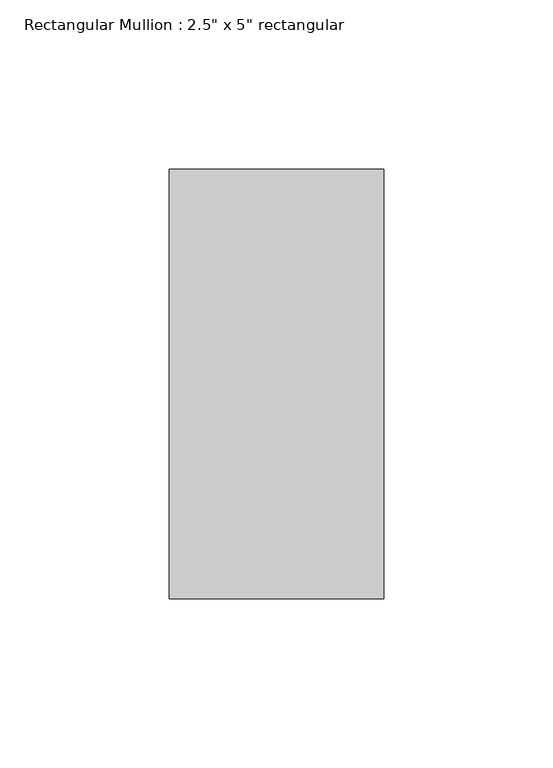
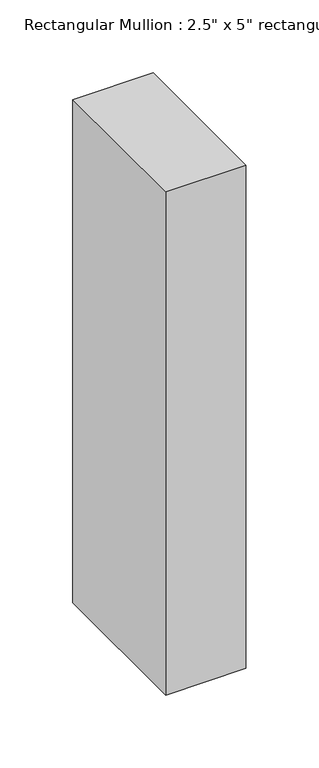
"""IFC4 building model written with IfcOpenShell, lengths in millimetres: member geometry."""

from ifc_helpers import new_model, si_unit, frame, origin, place, context, project, spatial, polyline, outline, extrude, source, transform, mapped, element, save


def member_b2da0656(model_context):
    return source(origin(), model_context, "Body", "SweptSolid", [
        extrude(outline(polyline([(0.0, 63.5), (0.0, -63.5), (-63.5, -63.5), (-63.5, 63.5), (0.0, 63.5)])), frame((0.0, 0.0, -421.2166667), z_axis=(0.0, 0.0, 1.0), x_axis=(1.0, 0.0, 0.0)), (0.0, 0.0, 1.0), 421.2166667),
    ])


if __name__ == "__main__":
    model = new_model("IFC4")
    model_context = context("Model", 3, world=origin())
    ifc_project = project(units=[si_unit("LENGTHUNIT", "METRE", prefix="MILLI")], contexts=[model_context])
    site = spatial("IfcSite", under=ifc_project)
    building = spatial("IfcBuilding", under=site)
    placement = place(None, origin())
    member_shape = member_b2da0656(model_context)
    element("IfcMember", 1, ObjectType="Rectangular Mullion : 2.5\" x 5\" rectangular", at=placement, inside=building, context=model_context, shape_type="MappedRepresentation", body=[
        mapped(member_shape, transform((0.0, 0.0, 0.0), x_axis=(1.0, 0.0, 0.0), y_axis=(0.0, 1.0, 0.0), z_axis=(0.0, 0.0, 1.0))),
    ])
    save(model, "model.ifc")

# Revit data of these elements
# Type "Rectangular Mullion : 2.5\" x 5\" rectangular"
#   built-in parameter 1007304 = 0.416667 (stored number, unit not read)
#   built-in parameter 1007301 = 0.104167 (stored number, unit not read)
#   built-in parameter 1007300 = 0.104167 (stored number, unit not read)
# Element 1 (IfcMember, "Rectangular Mullion : 2.5\" x 5\" rectangular")
#   Materials on its faces: "Aluminum"
# Materials
#   "Aluminum": class "Metal", colour RGB 247 247 247, transparency 0, Description = "Aluminum 6061", Cost = 0
